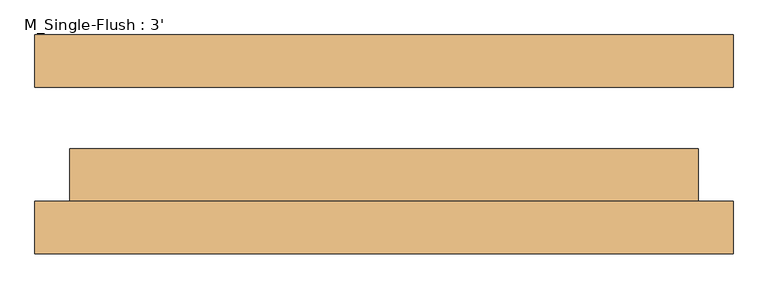
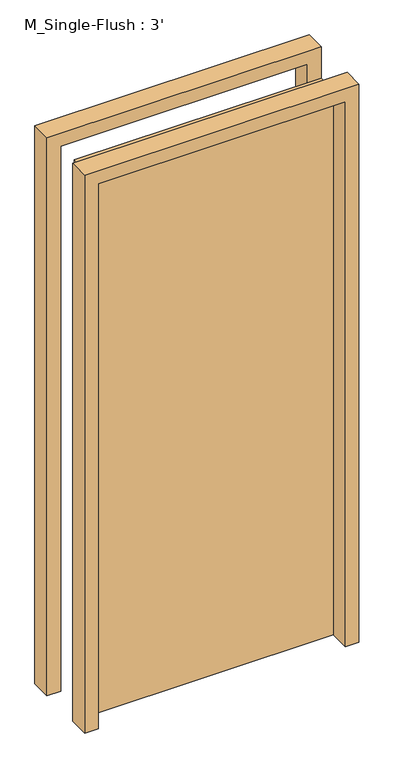
"""IFC4 building model written with IfcOpenShell, lengths in millimetres: door geometry, M_Single-Flush : 3'."""

from ifc_helpers import new_model, si_unit, frame, origin, origin_with_axes, place, context, project, spatial, polyline, outline, extrude, source, transform, mapped, element, save


def m_single_flush_3_86d08d0d(model_context):
    return source(origin(), model_context, "Body", "SweptSolid", [
        extrude(outline(polyline([(2184.4, -508.0), (0.0, -508.0), (0.0, -457.2), (2133.6, -457.2), (2133.6, 457.2), (0.0, 457.2), (0.0, 508.0), (2184.4, 508.0), (2184.4, -508.0)])), frame((0.0, -159.1, 0.0), z_axis=(0.0, 1.0, 0.0), x_axis=(0.0, 0.0, 1.0)), (0.0, 0.0, 1.0), 76.2),
        extrude(outline(polyline([(2184.4, 508.0), (2184.4, -508.0), (0.0, -508.0), (0.0, -457.2), (2133.6, -457.2), (2133.6, 457.2), (0.0, 457.2), (0.0, 508.0), (2184.4, 508.0)])), frame((0.0, 82.9, 0.0), z_axis=(0.0, 1.0, 0.0), x_axis=(0.0, 0.0, 1.0)), (0.0, 0.0, 1.0), 76.2),
        extrude(outline(polyline([(457.2, -6.7), (457.2, -82.9), (-457.2, -82.9), (-457.2, -6.7), (457.2, -6.7)])), origin_with_axes(), (0.0, 0.0, 1.0), 2133.6),
    ])


if __name__ == "__main__":
    model = new_model("IFC4")
    model_context = context("Model", 3, world=origin())
    ifc_project = project(units=[si_unit("LENGTHUNIT", "METRE", prefix="MILLI")], contexts=[model_context])
    site = spatial("IfcSite", under=ifc_project)
    building = spatial("IfcBuilding", under=site)
    placement = place(None, origin())
    m_single_flush_3_shape = m_single_flush_3_86d08d0d(model_context)
    element("IfcDoor", 1, ObjectType="M_Single-Flush : 3'", at=placement, inside=building, context=model_context, shape_type="MappedRepresentation", body=[
        mapped(m_single_flush_3_shape, transform((0.0, 0.0, 0.0), x_axis=(1.0, 0.0, 0.0), y_axis=(0.0, 1.0, 0.0), z_axis=(0.0, 0.0, 1.0))),
    ])
    save(model, "model.ifc")

# Revit data of these elements
# Type "M_Single-Flush : 3'"
#   Type Mark = "23"
#   Thickness = 0' - 3"
#   Height = 7' - 0"
#   Trim Projection Ext = 0' - 3"
#   Trim Projection Int = 0' - 3"
#   Trim Width = 0' - 2"
#   Width = 3' - 0"
#   Wall Closure = 2
#   Door Material = Door - Panel
#   Frame Material = Door - Panel
#   Function = (empty or 0)
# Element 1 (IfcDoor, "M_Single-Flush : 3'")
#   Materials on its faces: "Door - Panel"
# Materials
#   "Door - Panel": class "Wood", colour RGB 114 82 51, transparency 0
